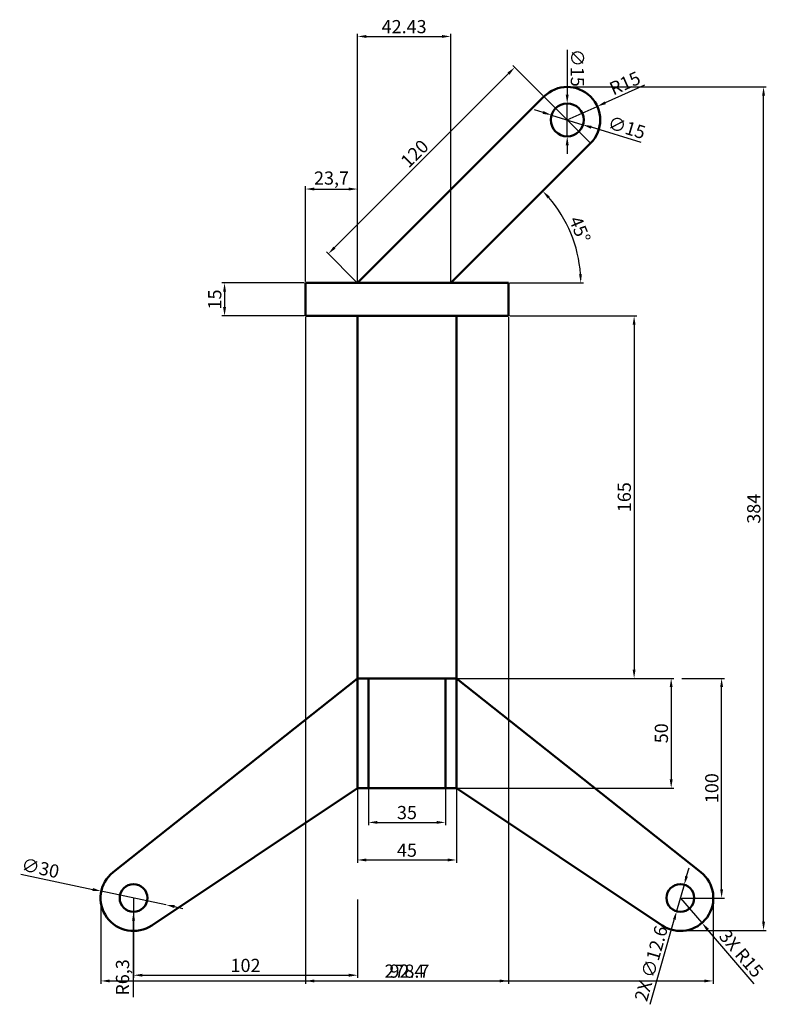
# Model space of a CAD drawing. Units: millimetres. Extents: x -29 to 311, y 102 to 550.
import ezdxf

# ---------------------------------------------------------------- set-up
doc = ezdxf.new("R2010")
doc.units = ezdxf.units.MM
for name, color, linetype, lineweight in [('M-CONS', 8, 'Continuous', 18), ('M-DIMS', 2, 'Continuous', 25), ('M-OUTL', 7, 'Continuous', 50)]:
    doc.layers.add(name, color=color, linetype=linetype, lineweight=lineweight)
doc.styles.get("Standard").update_dxf_attribs({"font": 'arial.ttf'})
doc.dimstyles.new('ISO-25', dxfattribs={"dimtxt": 6, "dimasz": 4, "dimexe": 1.25, "dimexo": 0.625, "dimtad": 1, "dimtxsty": 'Standard', "dimcen": 2.5, "dimadec": 0, "dimazin": 0, "dimtfac": 1, "dimtmove": 0, "dimatfit": 3, "dimfxl": 1, "dimarcsym": 0})

# ---------------------------------------------------------------- blocks, each defined once
blk = doc.blocks.new('*D1')
at = {"layer": 'Defpoints', "color": 0, "transparency": 16777216}
for p in [(130.22, 200.34), (165.22, 200.34), (165.22, 184.76)]:
    blk.add_point(p, dxfattribs=at)
at = {"layer": 'M-DIMS', "color": 0, "lineweight": -2, "transparency": 16777216}
for p, q in [((130.22, 199.72), (130.22, 183.51)), ((165.22, 199.72), (165.22, 183.51)), ((134.22, 184.76), (161.22, 184.76))]:
    blk.add_line(p, q, dxfattribs=at)
at = {"layer": 'M-DIMS', "color": 0, "transparency": 16777216}
for points in [[(134.22, 185.43), (134.22, 184.1), (130.22, 184.76)], [(161.22, 185.43), (161.22, 184.1), (165.22, 184.76)]]:
    blk.add_solid(points, dxfattribs=at)
at = {"layer": 'M-DIMS', "color": 0, "transparency": 16777216, "insert": (147.72, 188.46), "char_height": 6, "attachment_point": 5}
blk.add_mtext('35', dxfattribs=at)
blk = doc.blocks.new('*D2')
at = {"layer": 'Defpoints', "color": 0, "transparency": 16777216}
for p in [(125.22, 200.34), (170.22, 200.34), (170.22, 167.65)]:
    blk.add_point(p, dxfattribs=at)
at = {"layer": 'M-DIMS', "color": 0, "lineweight": -2, "transparency": 16777216}
for p, q in [((125.22, 199.72), (125.22, 166.4)), ((170.22, 199.72), (170.22, 166.4)), ((129.22, 167.65), (166.22, 167.65))]:
    blk.add_line(p, q, dxfattribs=at)
at = {"layer": 'M-DIMS', "color": 0, "transparency": 16777216}
for points in [[(129.22, 168.32), (129.22, 166.99), (125.22, 167.65)], [(166.22, 168.32), (166.22, 166.99), (170.22, 167.65)]]:
    blk.add_solid(points, dxfattribs=at)
at = {"layer": 'M-DIMS', "color": 0, "transparency": 16777216, "insert": (147.72, 171.33), "char_height": 6, "attachment_point": 5}
blk.add_mtext('45', dxfattribs=at)
blk = doc.blocks.new('*D3')
at = {"layer": 'Defpoints', "color": 0, "transparency": 16777216}
for p in [(170.22, 250.34), (170.22, 200.34), (268.02, 200.34)]:
    blk.add_point(p, dxfattribs=at)
at = {"layer": 'M-DIMS', "color": 0, "lineweight": -2, "transparency": 16777216}
for p, q in [((170.85, 250.34), (269.27, 250.34)), ((268.02, 246.34), (268.02, 204.34)), ((170.85, 200.34), (269.27, 200.34))]:
    blk.add_line(p, q, dxfattribs=at)
at = {"layer": 'M-DIMS', "color": 0, "transparency": 16777216}
for points in [[(267.36, 246.34), (268.69, 246.34), (268.02, 250.34)], [(267.36, 204.34), (268.69, 204.34), (268.02, 200.34)]]:
    blk.add_solid(points, dxfattribs=at)
at = {"layer": 'M-DIMS', "color": 0, "transparency": 16777216, "insert": (264.34, 225.34), "char_height": 6, "attachment_point": 5, "rotation": 90}
blk.add_mtext('50', dxfattribs=at)
blk = doc.blocks.new('*D4')
at = {"layer": 'Defpoints', "color": 0, "transparency": 16777216}
for p in [(193.92, 415.34), (193.92, 250.34), (251.14, 250.34)]:
    blk.add_point(p, dxfattribs=at)
at = {"layer": 'M-DIMS', "color": 0, "lineweight": -2, "transparency": 16777216}
for p, q in [((194.55, 415.34), (252.39, 415.34)), ((251.14, 411.34), (251.14, 254.34)), ((194.55, 250.34), (252.39, 250.34))]:
    blk.add_line(p, q, dxfattribs=at)
at = {"layer": 'M-DIMS', "color": 0, "transparency": 16777216}
for points in [[(250.47, 411.34), (251.81, 411.34), (251.14, 415.34)], [(250.47, 254.34), (251.81, 254.34), (251.14, 250.34)]]:
    blk.add_solid(points, dxfattribs=at)
at = {"layer": 'M-DIMS', "color": 0, "transparency": 16777216, "insert": (247.45, 332.84), "char_height": 6, "attachment_point": 5, "rotation": 90}
blk.add_mtext('165', dxfattribs=at)
blk = doc.blocks.new('*D5')
at = {"layer": 'Defpoints', "color": 0, "transparency": 16777216}
for p in [(8.54, 153.43), (37.9, 147.26)]:
    blk.add_point(p, dxfattribs=at)
at = {"layer": 'M-DIMS', "color": 0, "lineweight": -2, "transparency": 16777216}
for p, q in [((-28.14, 161.13), (4.63, 154.25)), ((37.9, 147.26), (8.54, 153.43)), ((41.82, 146.44), (45.73, 145.62))]:
    blk.add_line(p, q, dxfattribs=at)
at = {"layer": 'M-DIMS', "color": 0, "transparency": 16777216}
for points in [[(4.77, 154.9), (4.49, 153.6), (8.54, 153.43)], [(41.96, 147.09), (41.68, 145.79), (37.9, 147.26)]]:
    blk.add_solid(points, dxfattribs=at)
at = {"layer": 'M-DIMS', "color": 0, "transparency": 16777216, "insert": (-19.35, 163.23), "char_height": 6, "attachment_point": 5, "rotation": 348.1374}
blk.add_mtext('∅30', dxfattribs=at)
blk = doc.blocks.new('*D6')
at = {"layer": 'Defpoints', "color": 0, "transparency": 16777216}
for p in [(23.22, 150.34), (23.22, 144.04)]:
    blk.add_point(p, dxfattribs=at)
at = {"layer": 'M-DIMS', "color": 0, "lineweight": -2, "transparency": 16777216}
for p, q in [((23.22, 150.34), (23.22, 144.04)), ((23.22, 105.21), (23.22, 140.04))]:
    blk.add_line(p, q, dxfattribs=at)
at = {"layer": 'M-DIMS', "color": 0, "transparency": 16777216}
blk.add_solid([(22.56, 140.04), (23.89, 140.04), (23.22, 144.04)], dxfattribs=at)
at = {"layer": 'M-DIMS', "color": 0, "transparency": 16777216, "insert": (18.99, 114.17), "char_height": 6, "attachment_point": 5, "rotation": 90}
blk.add_mtext('R6,3', dxfattribs=at)
blk = doc.blocks.new('*D7')
at = {"layer": 'Defpoints', "color": 0, "transparency": 16777216}
for p in [(23.22, 150.34), (125.22, 150.34), (125.22, 115.18)]:
    blk.add_point(p, dxfattribs=at)
at = {"layer": 'M-DIMS', "color": 0, "lineweight": -2, "transparency": 16777216}
for p, q in [((23.22, 149.72), (23.22, 113.93)), ((125.22, 149.72), (125.22, 113.93)), ((27.22, 115.18), (121.22, 115.18))]:
    blk.add_line(p, q, dxfattribs=at)
at = {"layer": 'M-DIMS', "color": 0, "transparency": 16777216}
for points in [[(27.22, 115.85), (27.22, 114.52), (23.22, 115.18)], [(121.22, 115.85), (121.22, 114.52), (125.22, 115.18)]]:
    blk.add_solid(points, dxfattribs=at)
at = {"layer": 'M-DIMS', "color": 0, "transparency": 16777216, "insert": (74.22, 118.87), "char_height": 6, "attachment_point": 5}
blk.add_mtext('102', dxfattribs=at)
blk = doc.blocks.new('*D8')
at = {"layer": 'Defpoints', "color": 0, "transparency": 16777216}
for p in [(101.52, 430.34), (64.67, 415.34), (101.52, 415.34)]:
    blk.add_point(p, dxfattribs=at)
at = {"layer": 'M-DIMS', "color": 0, "lineweight": -2, "transparency": 16777216}
for p, q in [((100.9, 430.34), (63.42, 430.34)), ((64.67, 426.34), (64.67, 419.34)), ((100.9, 415.34), (63.42, 415.34))]:
    blk.add_line(p, q, dxfattribs=at)
at = {"layer": 'M-DIMS', "color": 0, "transparency": 16777216}
for points in [[(64, 426.34), (65.34, 426.34), (64.67, 430.34)], [(64, 419.34), (65.34, 419.34), (64.67, 415.34)]]:
    blk.add_solid(points, dxfattribs=at)
at = {"layer": 'M-DIMS', "color": 0, "transparency": 16777216, "insert": (60.98, 422.84), "char_height": 6, "attachment_point": 5, "rotation": 90}
blk.add_mtext('15', dxfattribs=at)
blk = doc.blocks.new('*D9')
at = {"layer": 'Defpoints', "color": 0, "transparency": 16777216}
for p in [(125.22, 473.11), (101.52, 430.34), (125.22, 430.34)]:
    blk.add_point(p, dxfattribs=at)
at = {"layer": 'M-DIMS', "color": 0, "lineweight": -2, "transparency": 16777216}
for p, q in [((101.52, 430.97), (101.52, 474.36)), ((105.52, 473.11), (121.22, 473.11)), ((125.22, 430.97), (125.22, 474.36))]:
    blk.add_line(p, q, dxfattribs=at)
at = {"layer": 'M-DIMS', "color": 0, "transparency": 16777216}
for points in [[(105.52, 473.78), (105.52, 472.45), (101.52, 473.11)], [(121.22, 473.78), (121.22, 472.45), (125.22, 473.11)]]:
    blk.add_solid(points, dxfattribs=at)
at = {"layer": 'M-DIMS', "color": 0, "transparency": 16777216, "insert": (113.37, 477.34), "char_height": 6, "attachment_point": 5}
blk.add_mtext('23,7', dxfattribs=at)
blk = doc.blocks.new('*D10')
at = {"layer": 'Defpoints', "color": 0, "transparency": 16777216}
for p in [(196.77, 528.5), (210.08, 515.2), (125.22, 430.34)]:
    blk.add_point(p, dxfattribs=at)
at = {"layer": 'M-DIMS', "color": 0, "lineweight": -2, "transparency": 16777216}
for p, q in [((209.64, 515.64), (195.89, 529.38)), ((114.75, 446.48), (193.94, 525.67)), ((124.78, 430.79), (111.04, 444.53))]:
    blk.add_line(p, q, dxfattribs=at)
at = {"layer": 'M-DIMS', "color": 0, "transparency": 16777216}
for points in [[(193.47, 526.14), (194.42, 525.2), (196.77, 528.5)], [(114.28, 446.95), (115.22, 446), (111.92, 443.65)]]:
    blk.add_solid(points, dxfattribs=at)
at = {"layer": 'M-DIMS', "color": 0, "transparency": 16777216, "insert": (151.74, 488.68), "char_height": 6, "attachment_point": 5, "rotation": 45}
blk.add_mtext('120', dxfattribs=at)
blk = doc.blocks.new('*D11')
at = {"layer": 'Defpoints', "color": 0, "transparency": 16777216}
for p in [(234.37, 510.74), (220.68, 504.59)]:
    blk.add_point(p, dxfattribs=at)
at = {"layer": 'M-DIMS', "color": 0, "lineweight": -2, "transparency": 16777216}
for p, q in [((255.92, 520.42), (238.01, 512.38)), ((220.68, 504.59), (234.37, 510.74))]:
    blk.add_line(p, q, dxfattribs=at)
at = {"layer": 'M-DIMS', "color": 0, "transparency": 16777216}
blk.add_solid([(237.74, 512.99), (238.29, 511.77), (234.37, 510.74)], dxfattribs=at)
at = {"layer": 'M-DIMS', "color": 0, "transparency": 16777216, "insert": (247.28, 520.59), "char_height": 6, "attachment_point": 5, "rotation": 24.1986}
blk.add_mtext('R15', dxfattribs=at)
blk = doc.blocks.new('*D12')
at = {"layer": 'Defpoints', "color": 0, "transparency": 16777216}
for p in [(213.51, 506.79), (227.85, 502.39)]:
    blk.add_point(p, dxfattribs=at)
at = {"layer": 'M-DIMS', "color": 0, "lineweight": -2, "transparency": 16777216}
for p, q in [((209.69, 507.96), (205.86, 509.13)), ((213.51, 506.79), (227.85, 502.39)), ((254.29, 494.29), (231.68, 501.22))]:
    blk.add_line(p, q, dxfattribs=at)
at = {"layer": 'M-DIMS', "color": 0, "transparency": 16777216}
for points in [[(209.88, 508.6), (209.49, 507.32), (213.51, 506.79)], [(231.87, 501.86), (231.48, 500.58), (227.85, 502.39)]]:
    blk.add_solid(points, dxfattribs=at)
at = {"layer": 'M-DIMS', "color": 0, "transparency": 16777216, "insert": (247.57, 500.38), "char_height": 6, "attachment_point": 5, "rotation": 342.9591}
blk.add_mtext('∅15', dxfattribs=at)
blk = doc.blocks.new('*D13')
at = {"layer": 'Defpoints', "color": 0, "transparency": 16777216}
for p in [(231.29, 493.98), (224.84, 445.67), (101.52, 430.34), (167.65, 430.34), (193.92, 430.34)]:
    blk.add_point(p, dxfattribs=at)
at = {"layer": 'M-DIMS', "color": 0, "lineweight": -2, "transparency": 16777216}
blk.add_line((194.55, 430.34), (228.11, 430.34), dxfattribs=at)
blk.add_arc((167.65, 430.34), 59.21, 3.8717, 41.1283, dxfattribs=at)
at = {"layer": 'M-DIMS', "color": 0, "transparency": 16777216}
for points in [[(211.76, 468.83), (212.73, 469.74), (209.52, 472.21)], [(227.39, 434.36), (226.06, 434.32), (226.86, 430.34)]]:
    blk.add_solid(points, dxfattribs=at)
at = {"layer": 'M-DIMS', "color": 0, "transparency": 16777216, "insert": (225.75, 454.41), "char_height": 6, "attachment_point": 5, "rotation": 292.5}
blk.add_mtext('45°', dxfattribs=at)
blk = doc.blocks.new('*D14')
at = {"layer": 'Defpoints', "color": 0, "transparency": 16777216}
for p in [(272.22, 250.34), (290.98, 250.34), (272.22, 150.34)]:
    blk.add_point(p, dxfattribs=at)
at = {"layer": 'M-DIMS', "color": 0, "lineweight": -2, "transparency": 16777216}
for p, q in [((272.85, 250.34), (292.23, 250.34)), ((290.98, 154.34), (290.98, 246.34)), ((272.85, 150.34), (292.23, 150.34))]:
    blk.add_line(p, q, dxfattribs=at)
at = {"layer": 'M-DIMS', "color": 0, "transparency": 16777216}
for points in [[(290.32, 246.34), (291.65, 246.34), (290.98, 250.34)], [(290.32, 154.34), (291.65, 154.34), (290.98, 150.34)]]:
    blk.add_solid(points, dxfattribs=at)
at = {"layer": 'M-DIMS', "color": 0, "transparency": 16777216, "insert": (287.29, 200.34), "char_height": 6, "attachment_point": 5, "rotation": 90}
blk.add_mtext('100', dxfattribs=at)
blk = doc.blocks.new('BRACKET-LOWER-ARM')
for p, q in [((0, 65), (0, 115)), ((111.32, 26.75), (0, 115)), ((93.68, 2.52), (0, 65))]:
    blk.add_line(p, q)
blk.add_circle((102, 15), 6.3)
blk.add_arc((102, 15), 15, 236.2982, 51.5951)
blk = doc.blocks.new('*D16')
at = {"layer": 'Defpoints', "color": 0, "transparency": 16777216}
for p in [(8.36, 152.37), (287.09, 152.37), (287.09, 112.58)]:
    blk.add_point(p, dxfattribs=at)
at = {"layer": 'M-DIMS', "color": 0, "lineweight": -2, "transparency": 16777216}
for p, q in [((8.36, 151.75), (8.36, 111.33)), ((287.09, 151.75), (287.09, 111.33)), ((12.36, 112.58), (283.09, 112.58))]:
    blk.add_line(p, q, dxfattribs=at)
at = {"layer": 'M-DIMS', "color": 0, "transparency": 16777216}
for points in [[(12.36, 113.24), (12.36, 111.91), (8.36, 112.58)], [(283.09, 113.24), (283.09, 111.91), (287.09, 112.58)]]:
    blk.add_solid(points, dxfattribs=at)
at = {"layer": 'M-DIMS', "color": 0, "transparency": 16777216, "insert": (147.72, 116.27), "char_height": 6, "attachment_point": 5}
blk.add_mtext('278.7', dxfattribs=at)
blk = doc.blocks.new('*D17')
at = {"layer": 'Defpoints', "color": 0, "transparency": 16777216}
for p in [(220.65, 519.59), (310.09, 519.59), (274.86, 135.58)]:
    blk.add_point(p, dxfattribs=at)
at = {"layer": 'M-DIMS', "color": 0, "lineweight": -2, "transparency": 16777216}
for p, q in [((221.28, 519.59), (311.34, 519.59)), ((310.09, 139.58), (310.09, 515.59)), ((275.49, 135.58), (311.34, 135.58))]:
    blk.add_line(p, q, dxfattribs=at)
at = {"layer": 'M-DIMS', "color": 0, "transparency": 16777216}
for points in [[(309.42, 515.59), (310.75, 515.59), (310.09, 519.59)], [(309.42, 139.58), (310.75, 139.58), (310.09, 135.58)]]:
    blk.add_solid(points, dxfattribs=at)
at = {"layer": 'M-DIMS', "color": 0, "transparency": 16777216, "insert": (306.4, 327.58), "char_height": 6, "attachment_point": 5, "rotation": 90}
blk.add_mtext('384', dxfattribs=at)
blk = doc.blocks.new('*D18')
at = {"layer": 'Defpoints', "color": 0, "transparency": 16777216}
for p in [(101.52, 415.34), (193.92, 415.34), (193.92, 112.58)]:
    blk.add_point(p, dxfattribs=at)
at = {"layer": 'M-DIMS', "color": 0, "lineweight": -2, "transparency": 16777216}
for p, q in [((101.52, 414.72), (101.52, 111.33)), ((193.92, 414.72), (193.92, 111.33)), ((105.52, 112.58), (189.92, 112.58))]:
    blk.add_line(p, q, dxfattribs=at)
at = {"layer": 'M-DIMS', "color": 0, "transparency": 16777216}
for points in [[(105.52, 113.24), (105.52, 111.91), (101.52, 112.58)], [(189.92, 113.24), (189.92, 111.91), (193.92, 112.58)]]:
    blk.add_solid(points, dxfattribs=at)
at = {"layer": 'M-DIMS', "color": 0, "transparency": 16777216, "insert": (147.72, 116.27), "char_height": 6, "attachment_point": 5}
blk.add_mtext('92.4', dxfattribs=at)
blk = doc.blocks.new('*D19')
at = {"layer": 'Defpoints', "color": 0, "transparency": 16777216}
for p in [(167.65, 542.59), (125.22, 430.34), (167.65, 430.34)]:
    blk.add_point(p, dxfattribs=at)
at = {"layer": 'M-DIMS', "color": 0, "lineweight": -2, "transparency": 16777216}
for p, q in [((125.22, 430.97), (125.22, 543.84)), ((129.22, 542.59), (163.65, 542.59)), ((167.65, 430.97), (167.65, 543.84))]:
    blk.add_line(p, q, dxfattribs=at)
at = {"layer": 'M-DIMS', "color": 0, "transparency": 16777216}
for points in [[(129.22, 543.26), (129.22, 541.92), (125.22, 542.59)], [(163.65, 543.26), (163.65, 541.92), (167.65, 542.59)]]:
    blk.add_solid(points, dxfattribs=at)
at = {"layer": 'M-DIMS', "color": 0, "transparency": 16777216, "insert": (146.44, 546.28), "char_height": 6, "attachment_point": 5}
blk.add_mtext('42.43', dxfattribs=at)
blk = doc.blocks.new('*D20')
at = {"layer": 'Defpoints', "color": 0, "transparency": 16777216}
for p in [(272.22, 150.34), (282.02, 138.98)]:
    blk.add_point(p, dxfattribs=at)
at = {"layer": 'M-DIMS', "color": 0, "lineweight": -2, "transparency": 16777216}
for p, q in [((272.22, 150.34), (282.02, 138.98)), ((305.86, 111.32), (284.63, 135.95))]:
    blk.add_line(p, q, dxfattribs=at)
at = {"layer": 'M-DIMS', "color": 0, "transparency": 16777216}
blk.add_solid([(285.13, 136.39), (284.12, 135.52), (282.02, 138.98)], dxfattribs=at)
at = {"layer": 'M-DIMS', "color": 0, "transparency": 16777216, "insert": (299.34, 124.53), "char_height": 6, "attachment_point": 5, "rotation": 310.7542}
blk.add_mtext('3X R15', dxfattribs=at)
blk = doc.blocks.new('*D21')
at = {"layer": 'Defpoints', "color": 0, "transparency": 16777216}
for p in [(220.68, 512.09), (220.69, 497.09)]:
    blk.add_point(p, dxfattribs=at)
at = {"layer": 'M-DIMS', "color": 0, "lineweight": -2, "transparency": 16777216}
for p, q in [((220.67, 536.51), (220.68, 516.09)), ((220.69, 497.09), (220.68, 512.09)), ((220.69, 493.09), (220.69, 489.09))]:
    blk.add_line(p, q, dxfattribs=at)
at = {"layer": 'M-DIMS', "color": 0, "transparency": 16777216}
for points in [[(221.34, 516.09), (220.01, 516.09), (220.68, 512.09)], [(221.36, 493.09), (220.02, 493.09), (220.69, 497.09)]]:
    blk.add_solid(points, dxfattribs=at)
at = {"layer": 'M-DIMS', "color": 0, "transparency": 16777216, "insert": (224.53, 528.3), "char_height": 6, "attachment_point": 5, "rotation": 270.0301}
blk.add_mtext('∅15', dxfattribs=at)
blk = doc.blocks.new('*D22')
at = {"layer": 'Defpoints', "color": 0, "transparency": 16777216}
for p in [(273.95, 156.4), (270.5, 144.29)]:
    blk.add_point(p, dxfattribs=at)
at = {"layer": 'M-DIMS', "color": 0, "lineweight": -2, "transparency": 16777216}
for p, q in [((275.05, 160.25), (276.15, 164.09)), ((273.95, 156.4), (270.5, 144.29)), ((258.41, 101.94), (269.4, 140.44))]:
    blk.add_line(p, q, dxfattribs=at)
at = {"layer": 'M-DIMS', "color": 0, "transparency": 16777216}
for points in [[(274.41, 160.43), (275.69, 160.06), (273.95, 156.4)], [(268.76, 140.62), (270.04, 140.26), (270.5, 144.29)]]:
    blk.add_solid(points, dxfattribs=at)
at = {"layer": 'M-DIMS', "color": 0, "transparency": 16777216, "insert": (259.65, 120.32), "char_height": 6, "attachment_point": 5, "rotation": 74.0733}
blk.add_mtext('2X ∅12.6', dxfattribs=at)

msp = doc.modelspace()

# ---------------------------------------------------------------- linework, layer by layer
at = {"layer": 'M-CONS'}
for p, q in [((210.077, 515.196), (231.291, 493.983)), ((125.225, 430.343), (155.225, 430.343)), ((147.725, 250.343), (165.225, 250.343))]:
    msp.add_line(p, q, dxfattribs=at)
at = {"layer": 'M-OUTL'}
for p, q in [((125.225, 430.343), (210.077, 515.196)), ((167.651, 430.343), (231.291, 493.983)), ((193.925, 430.343), (101.525, 430.343)), ((101.525, 430.343), (101.525, 415.343)), ((193.925, 415.343), (193.925, 430.343)), ((101.525, 415.343), (170.225, 415.343)), ((125.225, 415.343), (125.225, 250.343)), ((170.225, 250.343), (170.225, 415.343)), ((170.225, 415.343), (193.925, 415.343)), ((125.225, 250.343), (170.225, 250.343)), ((165.225, 250.343), (130.225, 250.343)), ((130.225, 250.343), (130.225, 200.343)), ((165.225, 200.343), (165.225, 250.343)), ((125.225, 200.343), (170.225, 200.343)), ((130.225, 200.343), (165.225, 200.343))]:
    msp.add_line(p, q, dxfattribs=at)
msp.add_circle((220.684, 504.59), 7.5, dxfattribs=at)
msp.add_arc((220.684, 504.59), 15, 315, 135, dxfattribs=at)

# ---------------------------------------------------------------- block references
at = {"layer": 'M-OUTL', "extrusion": (0, 0, -1), "zscale": -1}
msp.add_blockref('BRACKET-LOWER-ARM', (-125.224, 135.343), dxfattribs=at)
at = {"layer": 'M-OUTL'}
msp.add_blockref('BRACKET-LOWER-ARM', (170.225, 135.343), dxfattribs=at)

# ---------------------------------------------------------------- dimensions: what is measured, and where the dimension line sits
at = {"layer": 'M-DIMS'}
for base, p1, p2, override, picture, middle in [((167.651, 542.59), (125.225, 430.343), (167.651, 430.343), {"dimdec": 2, "dimlfac": 1, "dimrnd": 0, "dimzin": 0, "dimdsep": 46, "dimlunit": 2}, '*D19', (146.438, 546.28)), ((193.925, 112.577), (101.525, 415.343), (193.925, 415.343), {"dimdec": 1, "dimlfac": 1, "dimrnd": 0, "dimzin": 0, "dimdsep": 46, "dimlunit": 2}, '*D18', (147.725, 116.265)), ((170.225, 167.655), (125.225, 200.343), (170.225, 200.343), {"dimclrd": 0, "dimclre": 0, "dimclrt": 0}, '*D2', (147.725, 171.331)), ((165.225, 184.765), (130.225, 200.343), (165.225, 200.343), {"dimclrd": 0, "dimclre": 0, "dimclrt": 0}, '*D1', (147.725, 188.455)), ((287.087, 112.577), (8.362, 152.371), (287.087, 152.371), {"dimdec": 1, "dimlfac": 1, "dimrnd": 0, "dimzin": 0, "dimdsep": 46, "dimlunit": 2}, '*D16', (147.725, 116.265)), ((125.225, 115.182), (23.225, 150.343), (125.225, 150.343), {"dimclrd": 0, "dimclre": 0, "dimclrt": 0}, '*D7', (74.225, 118.871))]:
    dim = msp.add_linear_dim(base=base, p1=p1, p2=p2, dimstyle='ISO-25', override=override, dxfattribs=at)
    dim.commit()
    dim.dimension.update_dxf_attribs({"geometry": picture, "text_midpoint": middle})
dim = msp.add_diameter_dim_2p(p1=(220.688, 497.09), p2=(220.68, 512.09), dimstyle='ISO-25', override={"dimdec": 0, "dimlfac": 1, "dimrnd": 0, "dimzin": 0, "dimdsep": 46, "dimlunit": 2}, dxfattribs=at)
dim.commit()
dim.dimension.update_dxf_attribs({"geometry": '*D21', "text_midpoint": (220.671, 528.298)})
for p1, p2, distance, picture, middle in [((125.225, 430.343), (210.077, 515.196), 18.815, '*D10', (151.738, 488.682)), ((101.525, 430.343), (125.225, 430.343), 42.771, '*D9', (113.375, 477.345)), ((272.225, 150.343), (272.225, 250.343), -18.757, '*D14', (287.293, 200.343))]:
    dim = msp.add_aligned_dim(p1=p1, p2=p2, distance=distance, dimstyle='ISO-25', override={"dimclrd": 0, "dimclre": 0, "dimclrt": 0}, dxfattribs=at)
    dim.commit()
    dim.dimension.update_dxf_attribs({"geometry": picture, "text_midpoint": middle})
dim = msp.add_radius_dim(center=(220.684, 504.59), mpoint=(234.366, 510.738), dimstyle='ISO-25', override={"dimclrd": 0, "dimclre": 0, "dimclrt": 0}, dxfattribs=at)
dim.commit()
dim.dimension.update_dxf_attribs({"geometry": '*D11', "text_midpoint": (247.28, 520.585)})
for base, p1, p2, override, picture, middle in [((310.087, 519.59), (274.861, 135.577), (220.651, 519.59), {"dimdec": 0, "dimlfac": 1, "dimrnd": 0, "dimzin": 0, "dimdsep": 46, "dimlunit": 2}, '*D17', (306.396, 327.583)), ((64.67, 415.343), (101.525, 430.343), (101.525, 415.343), {"dimclrd": 0, "dimclre": 0, "dimclrt": 0}, '*D8', (60.981, 422.843)), ((251.139, 250.343), (193.925, 415.343), (193.925, 250.343), {"dimclrd": 0, "dimclre": 0, "dimclrt": 0}, '*D4', (247.45, 332.843)), ((268.024, 200.343), (170.225, 250.343), (170.225, 200.343), {"dimclrd": 0, "dimclre": 0, "dimclrt": 0}, '*D3', (264.336, 225.343))]:
    dim = msp.add_linear_dim(base=base, p1=p1, p2=p2, angle=90, dimstyle='ISO-25', override=override, dxfattribs=at)
    dim.commit()
    dim.dimension.update_dxf_attribs({"geometry": picture, "text_midpoint": middle})
for p1, p2, picture, middle in [((213.513, 506.787), (227.855, 502.392), '*D12', (246.437, 496.696)), ((37.904, 147.26), (8.545, 153.427), '*D5', (-20.142, 159.452))]:
    dim = msp.add_diameter_dim_2p(p1=p1, p2=p2, dimstyle='ISO-25', override={"dimclrd": 0, "dimclre": 0, "dimclrt": 0}, dxfattribs=at)
    dim.commit()
    dim.dimension.update_dxf_attribs({"geometry": picture, "text_midpoint": middle, "dimtype": 163})
dim = msp.add_angular_dim_2l(base=(224.84, 445.667), line1=((193.925, 430.343), (101.525, 430.343)), line2=((167.651, 430.343), (231.291, 493.983)), dimstyle='ISO-25', override={"dimclrd": 0, "dimclre": 0, "dimclrt": 0}, dxfattribs=at)
dim.commit()
dim.dimension.update_dxf_attribs({"geometry": '*D13', "text_midpoint": (225.747, 454.407)})
dim = msp.add_diameter_dim_2p(p1=(273.953, 156.401), p2=(270.496, 144.285), text='2X <>', dimstyle='ISO-25', override={"dimdec": 1, "dimlfac": 1, "dimrnd": 0, "dimzin": 0, "dimdsep": 46, "dimlunit": 2}, dxfattribs=at)
dim.commit()
dim.dimension.update_dxf_attribs({"geometry": '*D22', "text_midpoint": (263.356, 119.267), "dimtype": 163})
dim = msp.add_radius_dim(center=(23.225, 150.343), mpoint=(23.225, 144.043), dimstyle='ISO-25', override={"dimclrd": 0, "dimclre": 0, "dimclrt": 0}, dxfattribs=at)
dim.commit()
dim.dimension.update_dxf_attribs({"geometry": '*D6', "text_midpoint": (23.225, 114.171), "dimtype": 164})
dim = msp.add_radius_dim(center=(272.225, 150.343), mpoint=(282.017, 138.981), text='3X <>', dimstyle='ISO-25', override={"dimdec": 0, "dimlfac": 1, "dimrnd": 0, "dimzin": 0, "dimdsep": 46, "dimlunit": 2}, dxfattribs=at)
dim.commit()
dim.dimension.update_dxf_attribs({"geometry": '*D20', "text_midpoint": (299.344, 124.527)})

doc.saveas('drawing.dxf')
